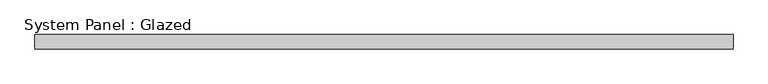
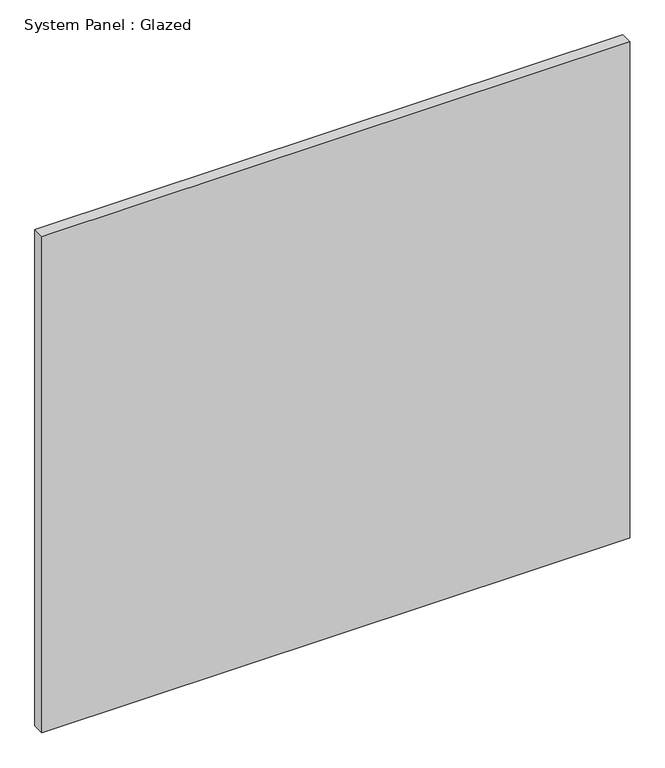
"""IFC4 building model written with IfcOpenShell, lengths in millimetres: plate geometry, System Panel : Glazed."""

from ifc_helpers import new_model, si_unit, origin, origin_with_axes, place, context, project, spatial, polyline, outline, extrude, source, transform, mapped, element, save


def system_panel_glazed_ffa60984(model_context):
    return source(origin(), model_context, "Body", "SweptSolid", [
        extrude(outline(polyline([(611.3911622, 19.05), (-611.3911622, 19.05), (-611.3911622, 44.45), (611.3911622, 44.45), (611.3911622, 19.05)])), origin_with_axes(), (0.0, 0.0, 1.0), 1092.2),
    ])


if __name__ == "__main__":
    model = new_model("IFC4")
    model_context = context("Model", 3, world=origin())
    ifc_project = project(units=[si_unit("LENGTHUNIT", "METRE", prefix="MILLI")], contexts=[model_context])
    site = spatial("IfcSite", under=ifc_project)
    building = spatial("IfcBuilding", under=site)
    placement = place(None, origin())
    system_panel_glazed_shape = system_panel_glazed_ffa60984(model_context)
    element("IfcPlate", 1, ObjectType="System Panel : Glazed", at=placement, inside=building, context=model_context, shape_type="MappedRepresentation", body=[
        mapped(system_panel_glazed_shape, transform((0.0, 0.0, 0.0), x_axis=(1.0, 0.0, 0.0), y_axis=(0.0, 1.0, 0.0), z_axis=(0.0, 0.0, 1.0))),
    ])
    save(model, "model.ifc")

# Revit data of these elements
# Type "System Panel : Glazed"
#   Construction Type Id = "GSP4R"
#   Analytic Construction = "1/8 in Pilkington single glazing"
#   Visual Light Transmittance = 0.9
#   Solar Heat Gain Coefficient = 0.86
#   Heat Transfer Coefficient (U) = 1.18115 BTU/(h·ft²·°F)
#   Define Thermal Properties by = 1
# Element 1 (IfcPlate, "System Panel : Glazed")
#   Materials on its faces: "Glass"
# Materials
#   "Glass": class "Glass", colour RGB 0 128 192, transparency 0.75, Description = "Soda Lime Glass", Cost = 0
